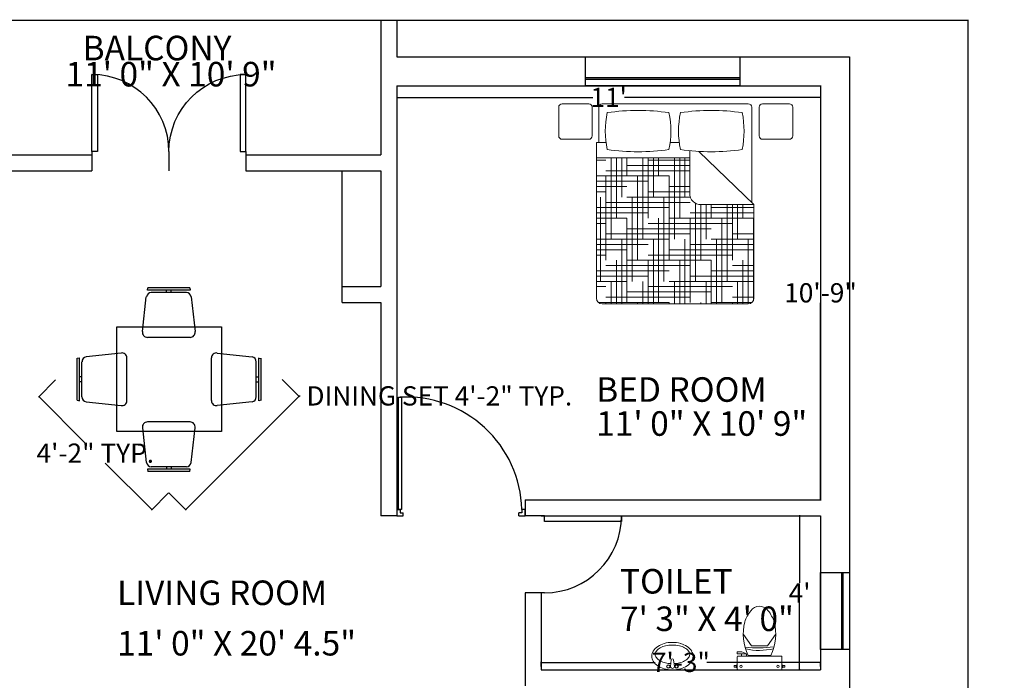
# Model space of a CAD drawing. Units: inches. Extents: x -113 to 5399, y -1393 to 3302.
# Tile 18 of 40: x 1779 to 2086, y 592 to 798. Entities that reach past the tile are written whole.
import ezdxf

# ---------------------------------------------------------------- set-up
doc = ezdxf.new("R2010")
doc.units = ezdxf.units.IN
doc.header["$MEASUREMENT"] = 0
for name, color, linetype, lineweight in [('A-ANNO-DIMS', 254, 'Continuous', 18), ('A-AREA-IDEN', 4, 'Continuous', 18), ('A-FLOR-FIXT', 8, 'Continuous', 18), ('doors', 2, 'Continuous', 25), ('furniture', 131, 'Continuous', 18), ('walls', 1, 'Continuous', 25), ('windows', 3, 'Continuous', 25)]:
    doc.layers.add(name, color=color, linetype=linetype, lineweight=lineweight)
doc.layers.add('B-FURNITURE', color=22, linetype='Continuous')
doc.styles.get("Standard").update_dxf_attribs({"font": 'arial.ttf'})
doc.dimstyles.get("Standard").update_dxf_attribs({"dimtxt": 6, "dimasz": 0.18, "dimexe": 0.18, "dimexo": 0.0625, "dimgap": 0.09, "dimtad": 0, "dimtih": 1, "dimtoh": 1, "dimdec": 1, "dimzin": 0, "dimdsep": 46, "dimlunit": 4, "dimtxsty": 'Standard', "dimblk": 'ARCHTICK', "dimcen": 0.09, "dimadec": 0, "dimazin": 0, "dimtfac": 1, "dimtdec": 1, "dimtofl": 0, "dimtmove": 0, "dimatfit": 3, "dimfxl": 1, "dimtolj": 1, "dimtzin": 0, "dimarcsym": 0})

# ---------------------------------------------------------------- blocks, each defined once
blk = doc.blocks.new('*U2')
for p, q in [((0, 0), (0, -6)), ((24, 0), (24, -6))]:
    blk.add_line(p, q)
blk.add_lwpolyline([(0, 0), (0, 24), (1.75, 24), (1.75, 0)], close=True)
blk.add_arc((0, 0), 24, 0, 90)
blk = doc.blocks.new('*X4')
at = {"color": 0}
for p, q in [((4.3594, 18.5625), (4.3594, 18.6457)), ((4.5, 18), (4.5, 18.6457)), ((4.5469, 18.1875), (4.5469, 18.6457)), ((4.5938, 18.375), (4.5938, 18.6457)), ((4.6406, 18.5625), (4.6406, 18.6457)), ((4.6875, 18.6094), (5.4375, 18.6094)), ((4.7812, 18), (4.7812, 18.6457)), ((4.8281, 18.1875), (4.8281, 18.6457)), ((4.875, 18.375), (4.875, 18.6457)), ((4.9219, 18.5625), (4.9219, 18.6457)), ((5.0625, 18), (5.0625, 18.6457)), ((5.1094, 18.1875), (5.1094, 18.6457)), ((5.1562, 18.375), (5.1562, 18.6457)), ((5.2031, 18.5625), (5.2031, 18.6457)), ((5.3438, 18), (5.3438, 18.6457)), ((5.3906, 18.1875), (5.3906, 18.6457)), ((5.4375, 18.375), (5.4375, 18.6457)), ((5.4844, 18.5625), (5.4844, 18.6457)), ((5.625, 18), (5.625, 18.6287)), ((4.3395, 18.5156), (5.0625, 18.5156)), ((4.4531, 17.8169), (4.4531, 18.5625)), ((4.5, 18.5625), (5.25, 18.5625)), ((4.7344, 17.8125), (4.7344, 18.5625)), ((5.0156, 17.8125), (5.0156, 18.5625)), ((5.2969, 17.8125), (5.2969, 18.5625)), ((5.4375, 18.5156), (5.6375, 18.5156)), ((5.5781, 17.8125), (5.5781, 18.5625)), ((5.625, 18.5625), (5.6375, 18.5625)), ((4.3395, 18.4688), (4.875, 18.4688)), ((4.3395, 18.4219), (4.6875, 18.4219)), ((5.0625, 18.4219), (5.6375, 18.4219)), ((5.25, 18.4688), (5.6375, 18.4688)), ((4.3395, 18.375), (4.5, 18.375)), ((4.4062, 17.8169), (4.4062, 18.375)), ((4.6875, 17.8114), (4.6875, 18.375)), ((4.6875, 18.3281), (5.4375, 18.3281)), ((4.875, 18.375), (5.625, 18.375)), ((4.9688, 17.625), (4.9688, 18.375)), ((5.25, 17.625), (5.25, 18.375)), ((5.5312, 17.625), (5.5312, 18.375)), ((4.3395, 18.2344), (5.0625, 18.2344)), ((4.5, 18.2812), (5.25, 18.2812)), ((5.4375, 18.2344), (5.6375, 18.2344)), ((5.625, 18.2812), (5.6375, 18.2812)), ((4.3395, 18.1875), (4.875, 18.1875)), ((4.3395, 18.1406), (4.6875, 18.1406)), ((4.3594, 17.8169), (4.3594, 18.1875)), ((4.6406, 17.8169), (4.6406, 18.1875)), ((4.9219, 17.4375), (4.9219, 18.1875)), ((5.0625, 18.1406), (5.6375, 18.1406)), ((5.2031, 17.4375), (5.2031, 18.1875)), ((5.25, 18.1875), (5.6375, 18.1875)), ((5.4844, 17.4375), (5.4844, 18.1875)), ((4.3395, 18.0938), (4.5, 18.0938)), ((4.6875, 18.0469), (5.4375, 18.0469)), ((4.875, 18.0938), (5.625, 18.0938)), ((4.5, 18), (5.25, 18)), ((4.5938, 17.8169), (4.5938, 18)), ((4.875, 17.25), (4.875, 18)), ((5.1562, 17.25), (5.1562, 18)), ((5.4375, 17.25), (5.4375, 18)), ((5.625, 18), (5.6375, 18)), ((4.3395, 17.9531), (5.0625, 17.9531)), ((4.3395, 17.9062), (4.875, 17.9062)), ((5.25, 17.9062), (5.6375, 17.9062)), ((5.4375, 17.9531), (5.6375, 17.9531)), ((4.3395, 17.8594), (4.6875, 17.8594)), ((4.8281, 17.2457), (4.8281, 17.8125)), ((4.875, 17.8125), (5.625, 17.8125)), ((5.0625, 17.8594), (5.6375, 17.8594)), ((5.1094, 17.2457), (5.1094, 17.8125)), ((5.3906, 17.2457), (5.3906, 17.8125)), ((4.7421, 17.7656), (5.4375, 17.7656)), ((4.7548, 17.7188), (5.25, 17.7188)), ((5.625, 17.7188), (5.6375, 17.7188)), ((4.7548, 17.6719), (5.0625, 17.6719)), ((4.7548, 17.625), (4.875, 17.625)), ((4.7812, 17.2457), (4.7812, 17.625)), ((5.0625, 17.2457), (5.0625, 17.625)), ((5.25, 17.625), (5.6375, 17.625)), ((5.3438, 17.2457), (5.3438, 17.625)), ((5.4375, 17.6719), (5.6375, 17.6719)), ((5.625, 17.2627), (5.625, 17.625)), ((4.875, 17.5312), (5.625, 17.5312)), ((5.0625, 17.5781), (5.6375, 17.5781)), ((4.7548, 17.4844), (5.4375, 17.4844)), ((4.7548, 17.4375), (5.25, 17.4375)), ((5.0156, 17.2457), (5.0156, 17.4375)), ((5.2969, 17.2457), (5.2969, 17.4375)), ((5.5781, 17.2457), (5.5781, 17.4375)), ((5.625, 17.4375), (5.6375, 17.4375)), ((4.7548, 17.3906), (5.0625, 17.3906)), ((4.7548, 17.3438), (4.875, 17.3438)), ((5.25, 17.3438), (5.6375, 17.3438)), ((5.4375, 17.3906), (5.6375, 17.3906)), ((5.0625, 17.2969), (5.6375, 17.2969)), ((4.875, 17.25), (5.6077, 17.25)), ((4.9688, 17.2457), (4.9688, 17.25)), ((5.25, 17.2457), (5.25, 17.25)), ((5.5312, 17.2457), (5.5312, 17.25))]:
    blk.add_line(p, q, dxfattribs=at)
blk = doc.blocks.new('MAT-P01')
for p, q in [((-0.0213, 0.8164), (-0.0213, 0.5605)), ((0.0087, 0.8464), (0.2471, 0.8464)), ((0.2771, 0.8164), (0.2771, 0.5605)), ((0.3437, 0.8164), (0.3437, -0.0316)), ((0.3737, 0.8464), (1.6737, 0.8464)), ((1.7037, 0.8164), (1.7037, 0.5005)), ((1.7622, 0.8164), (1.7622, 0.5605)), ((1.7922, 0.8464), (2.0306, 0.8464)), ((2.0606, 0.8164), (2.0606, 0.5605)), ((0.0087, 0.5305), (0.2471, 0.5305)), ((1.7922, 0.5305), (2.0306, 0.5305)), ((0.9879, 0.5005), (1.0693, 0.5005)), ((1.6393, 0.5005), (1.7237, 0.5005)), ((1.7237, 0.5005), (1.7237, -0.8836)), ((0.8146, 0.423), (0.3237, -0.0509)), ((0.8949, 0.4293), (0.8949, 0.0491)), ((0.8949, 0.3643), (1.7237, 0.3643)), ((0.8949, 0.3643), (0.8949, 0.0491)), ((0.8949, 0.3643), (1.7237, 0.3643)), ((1.7237, 0.3643), (1.7237, -0.8836)), ((0.3237, -0.0509), (0.7949, -0.0509)), ((0.3237, -0.0509), (0.3237, -0.8836)), ((0.3737, -0.9336), (1.6737, -0.9336))]:
    blk.add_line(p, q)
for centre, radius, start, end in [((0.0087, 0.8164), 0.03, 90, 180), ((0.2471, 0.8164), 0.03, 0, 90), ((0.3737, 0.8164), 0.03, 90, 180), ((1.6737, 0.8164), 0.03, 0, 90), ((1.7922, 0.8164), 0.03, 90, 180), ((2.0306, 0.8164), 0.03, 0, 90), ((1.2251, 0.6034), 0.8138, 168.37298, 191.62702), ((0.7029, -1.1436), 1.9306, 81.81622, 98.18378), ((0.1806, 0.6034), 0.8138, 348.37298, 11.62702), ((1.8766, 0.6034), 0.8138, 168.37298, 191.62702), ((1.3543, -1.1436), 1.9306, 81.81622, 98.18378), ((0.8321, 0.6034), 0.8138, 348.37298, 11.62702), ((0.0087, 0.5605), 0.03, 180, 270), ((0.2471, 0.5605), 0.03, 270, 0), ((1.7922, 0.5605), 0.03, 180, 270), ((2.0306, 0.5605), 0.03, 270, 0), ((0.7029, 2.3504), 1.9306, 261.81622, 278.18378), ((1.3543, 2.3504), 1.9306, 261.81622, 278.18378), ((0.7949, 0.0491), 0.1, 270, 0), ((0.3737, -0.8836), 0.05, 180, 270), ((1.6737, -0.8836), 0.05, 270, 0)]:
    blk.add_arc(centre, radius, start, end)
at = {"rotation": 270}
blk.add_blockref('*X4', (-16.9221, 4.7038), dxfattribs=at)
blk = doc.blocks.new('A$C6ACA79D1')
at = {"layer": 'B-FURNITURE'}
for p, q in [((-0.5034, 0.0535), (-0.8012, -0.2442)), ((-0.4835, 0.0392), (-0.7869, -0.2642)), ((-0.5034, 0.0535), (-0.4835, 0.0392)), ((-0.4291, 0.0003), (-0.1547, -0.2204)), ((0.7869, -0.259), (0.4835, 0.0444)), ((0.4842, 0.0434), (0.5041, 0.0577)), ((0.7427, -0.249), (0.4935, 0.0002)), ((0.8012, -0.239), (0.5034, 0.0587)), ((-0.4935, -0.005), (-0.7427, -0.2542)), ((-0.601, -0.1125), (-0.6181, -0.0954)), ((0.601, -0.1073), (0.6181, -0.0902)), ((-0.6352, -0.1467), (-0.6523, -0.1296)), ((0.6352, -0.1415), (0.6523, -0.1244)), ((-0.7859, -0.2635), (-0.8002, -0.2436)), ((0.4513, -0.594), (0.1485, -0.2912)), ((0.8012, -0.239), (0.7869, -0.259)), ((-0.1485, -0.2964), (-0.4513, -0.5992)), ((0.748, -0.3133), (0.5273, -0.5877)), ((-0.1485, -1.1937), (-0.4513, -0.8909)), ((0.4513, -0.8961), (0.1485, -1.199)), ((0.748, -1.1768), (0.5273, -0.9024)), ((-0.5034, -1.5436), (-0.8012, -1.2459)), ((-0.7859, -1.2266), (-0.8002, -1.2466)), ((-0.4835, -1.5293), (-0.7869, -1.226)), ((-0.4935, -1.4851), (-0.7427, -1.236)), ((-0.4291, -1.4904), (-0.1547, -1.2698)), ((0.7869, -1.2312), (0.4835, -1.5346)), ((0.7427, -1.2412), (0.4935, -1.4903)), ((0.8012, -1.2511), (0.5034, -1.5488)), ((0.8012, -1.2511), (0.7869, -1.2312)), ((-0.6352, -1.3434), (-0.6523, -1.3605)), ((-0.601, -1.3776), (-0.6181, -1.3948)), ((0.6352, -1.3486), (0.6523, -1.3657)), ((0.601, -1.3829), (0.6181, -1.4)), ((-0.5034, -1.5436), (-0.4835, -1.5293)), ((0.4842, -1.5336), (0.5041, -1.5478))]:
    blk.add_line(p, q, dxfattribs=at)
at = {"layer": 'B-FURNITURE', "ltscale": 300}
for p, q in [((0.1547, -0.2152), (0.4291, 0.0055)), ((-0.5273, -0.593), (-0.748, -0.3186)), ((-0.5273, -0.8972), (-0.748, -1.1716)), ((0.1547, -1.275), (0.4291, -1.4956))]:
    blk.add_line(p, q, dxfattribs=at)
blk.add_lwpolyline([(-0.7425, -0.7425), (0, 0), (0.7425, -0.7425), (0, -1.4849)], close=True, dxfattribs=at)
at = {"layer": 'B-FURNITURE', "ltscale": 400}
for centre, start, end in [((-0.4582, -0.0403), 54.40695, 135), ((0.4589, -0.0361), 45, 125.59305), ((-0.7063, -0.2888), 135, 215.59305), ((0.7073, -0.2843), 324.40695, 45), ((-0.7063, -1.2013), 144.40695, 225), ((0.7073, -1.2059), 315, 35.59305), ((-0.4582, -1.4498), 225, 305.59305), ((0.4589, -1.454), 234.40695, 315)]:
    blk.add_arc(centre, 0.0499, start, end, dxfattribs=at)
at = {"layer": 'B-FURNITURE', "ltscale": 300}
for centre, start, end in [((-0.1838, -0.261), 315, 54.40695), ((0.1838, -0.2558), 125.59305, 225), ((0.4866, -0.5586), 225, 324.40695), ((-0.4866, -0.5639), 215.59305, 315), ((-0.4866, -0.9263), 45, 144.40695), ((0.4866, -0.9315), 35.59305, 135), ((-0.1838, -1.2291), 305.59305, 45), ((0.1838, -1.2343), 135, 234.40695)]:
    blk.add_arc(centre, 0.05, start, end, dxfattribs=at)
blk = doc.blocks.new('toilet-3')
at = {"color": 0, "linetype": 'ByBlock'}
for p, q in [((-0.281, -0.05), (-0.281, -0.069)), ((-0.281, -0.05), (-0.261, -0.05)), ((-0.281, -0.069), (-0.261, -0.069)), ((-0.261, -0.047), (-0.261, -0.072)), ((-0.261, -0.047), (-0.251, -0.047)), ((-0.261, -0.072), (-0.251, -0.072)), ((-0.251, -0.047), (-0.251, -0.072)), ((-0.25, -0.03), (-0.25, -0.165)), ((0.24, -0.02), (-0.24, -0.02)), ((0.25, -0.03), (0.25, -0.165)), ((0.261, -0.047), (0.251, -0.047)), ((0.251, -0.047), (0.251, -0.072)), ((0.261, -0.072), (0.251, -0.072)), ((0.261, -0.047), (0.261, -0.072)), ((0.281, -0.05), (0.261, -0.05)), ((0.281, -0.069), (0.261, -0.069)), ((0.281, -0.05), (0.281, -0.069)), ((-0.144, -0.2), (-0.25, -0.2)), ((-0.25, -0.2), (-0.25, -0.222)), ((0.24, -0.175), (-0.24, -0.175)), ((-0.202, -0.2), (-0.202, -0.175)), ((-0.198, -0.222), (-0.16, -0.207)), ((-0.16, -0.207), (-0.16, -0.2)), ((-0.144, -0.2), (-0.144, -0.175)), ((0.125, -0.182), (-0.125, -0.182)), ((-0.198, -0.222), (-0.25, -0.222)), ((-0.089, -0.287), (-0.18, -0.415)), ((0.089, -0.287), (-0.089, -0.287)), ((0.089, -0.287), (0.18, -0.415))]:
    blk.add_line(p, q, dxfattribs=at)
for centre in [(-0.205, -0.059), (0.205, -0.059)]:
    blk.add_circle(centre, 0.0125, dxfattribs=at)
for centre, radius, start, end in [((-0.24, -0.03), 0.01, 90, 180), ((0.24, -0.03), 0.01, 0, 90), ((-0.24, -0.165), 0.01, 180, 270), ((0.376, -0.424), 0.557, 154.2321, 193.6755), ((-0.376, -0.424), 0.557, 346.3245, 25.7679), ((0.24, -0.165), 0.01, 270, 0), ((-0.013, -1.787), 1.521, 83.4552, 95.5271), ((-0.005, -0.896), 0.659, 75.9276, 103.0204), ((0.262, -0.406), 0.452, 199.2942, 217.2549), ((-0.265, -0.4), 0.457, 322.2382, 340.1051), ((-0.001, -0.609), 0.12, 216.3794, 323.6206)]:
    blk.add_arc(centre, radius, start, end, dxfattribs=at)
blk = doc.blocks.new('wash-6')
at = {"color": 0, "linetype": 'ByBlock'}
for p, q in [((-0.036, -0.063), (-0.021, -0.18)), ((0.036, -0.063), (0.021, -0.18))]:
    blk.add_line(p, q, dxfattribs=at)
for centre, radius in [((-0.075, -0.062), 0.0325), ((-0.075, -0.062), 0.0263), ((0.075, -0.062), 0.0325), ((0.075, -0.062), 0.0263)]:
    blk.add_circle(centre, radius, dxfattribs=at)
for centre, radius, start, end in [((0, -0.56), 0.56, 90, 105.4371), ((-0.204, -0.25), 0.17, 148.1465, 180), ((-0.107, -0.311), 0.285, 123.6901, 148.1465), ((-0.114, -0.361), 0.225, 118.369, 142.5096), ((-0.042, -0.407), 0.401, 105.4371, 123.6901), ((-0.045, -0.488), 0.37, 102.6081, 118.369), ((0, -0.69), 0.576, 92.9466, 102.6081), ((0, -0.063), 0.0361, 0, 180), ((0, -0.56), 0.56, 74.5629, 90), ((0, -0.69), 0.576, 77.3919, 87.0534), ((0.045, -0.488), 0.37, 61.631, 77.3919), ((0.042, -0.407), 0.401, 56.3099, 74.5629), ((0.114, -0.361), 0.225, 37.4904, 61.631), ((0.107, -0.311), 0.285, 31.8535, 56.3099), ((0.204, -0.25), 0.17, 0, 31.8535), ((-0.204, -0.25), 0.17, 180, 211.8535), ((-0.107, -0.189), 0.285, 211.8535, 236.3099), ((-0.217, -0.282), 0.0954, 142.5096, 180), ((-0.217, -0.282), 0.0954, 180, 217.4904), ((-0.114, -0.203), 0.225, 217.4904, 241.631), ((0, -0.18), 0.0215, 180, 0), ((0.114, -0.203), 0.225, 298.369, 322.5096), ((0.107, -0.189), 0.285, 303.6901, 328.1465), ((0.217, -0.282), 0.0954, 0, 37.4904), ((0.217, -0.282), 0.0954, 322.5096, 0), ((0.204, -0.25), 0.17, 328.1465, 0), ((-0.042, -0.092), 0.401, 236.3099, 254.5629), ((-0.045, -0.076), 0.37, 241.631, 257.3919), ((0, 0.06), 0.56, 254.5629, 270), ((0, 0.125), 0.576, 257.3919, 270), ((0, 0.125), 0.576, 270, 282.6081), ((0, 0.06), 0.56, 270, 285.4371), ((0.045, -0.076), 0.37, 282.6081, 298.369), ((0.042, -0.092), 0.401, 285.4371, 303.6901)]:
    blk.add_arc(centre, radius, start, end, dxfattribs=at)
blk = doc.blocks.new('_ArchTick')
at = {"color": 0, "linetype": 'ByBlock', "const_width": 0.15}
blk.add_lwpolyline([(-0.5, -0.5), (0.5, 0.5)], dxfattribs=at)
blk = doc.blocks.new('*D49')
at = {"layer": 'A-ANNO-DIMS', "color": 0, "lineweight": -2, "transparency": 16777216}
for p, q in [((2025.46, 777.53), (2028.44, 777.53)), ((2028.26, 777.53), (2028.26, 716.19)), ((2028.26, 648.53), (2028.26, 709.88)), ((2025.46, 648.53), (2028.44, 648.53))]:
    blk.add_line(p, q, dxfattribs=at)
at = {"layer": 'Defpoints', "color": 0, "transparency": 16777216}
for p in [(2025.39, 777.53), (2025.39, 648.53), (2028.26, 648.53)]:
    blk.add_point(p, dxfattribs=at)
at = {"layer": 'A-ANNO-DIMS', "color": 0, "lineweight": -2, "transparency": 16777216, "xscale": 0.18, "yscale": 0.18, "zscale": 0.18}
for p, rotation in [((2028.26, 777.53), 90), ((2028.26, 648.53), 270)]:
    blk.add_blockref('_ArchTick', p, dxfattribs=dict(at, rotation=rotation))
at = {"layer": 'A-ANNO-DIMS', "color": 0, "transparency": 16777216, "insert": (2028.26, 713.03), "char_height": 6, "attachment_point": 5}
blk.add_mtext('\\A1;10\'-9"', dxfattribs=at)
blk = doc.blocks.new('*D50')
at = {"layer": 'A-ANNO-DIMS', "color": 0, "lineweight": -2, "transparency": 16777216}
for p, q in [((1896.26, 773.9), (1957.36, 773.9)), ((1896.26, 773.84), (1896.26, 773.72)), ((2028.26, 773.9), (1967.16, 773.9)), ((2028.26, 773.96), (2028.26, 774.08))]:
    blk.add_line(p, q, dxfattribs=at)
at = {"layer": 'Defpoints', "color": 0, "transparency": 16777216}
for p in [(1896.26, 773.9), (2028.26, 773.9), (2028.26, 773.9)]:
    blk.add_point(p, dxfattribs=at)
at = {"layer": 'A-ANNO-DIMS', "color": 0, "lineweight": -2, "transparency": 16777216, "xscale": 0.18, "yscale": 0.18, "zscale": 0.18, "rotation": 180}
blk.add_blockref('_ArchTick', (1896.26, 773.9), dxfattribs=at)
at = {"layer": 'A-ANNO-DIMS', "color": 0, "lineweight": -2, "transparency": 16777216, "xscale": 0.18, "yscale": 0.18, "zscale": 0.18}
blk.add_blockref('_ArchTick', (2028.26, 773.9), dxfattribs=at)
at = {"layer": 'A-ANNO-DIMS', "color": 0, "transparency": 16777216, "insert": (1962.26, 773.9), "char_height": 6, "attachment_point": 5}
blk.add_mtext("\\A1;11'", dxfattribs=at)
blk = doc.blocks.new('*D51')
at = {"layer": 'A-ANNO-DIMS', "color": 0, "lineweight": -2, "transparency": 16777216}
for p, q in [((2021.92, 643.53), (2021.57, 643.53)), ((2021.75, 643.53), (2021.75, 622.62)), ((2021.75, 595.53), (2021.75, 616.44)), ((2021.92, 595.53), (2021.57, 595.53))]:
    blk.add_line(p, q, dxfattribs=at)
at = {"layer": 'Defpoints', "color": 0, "transparency": 16777216}
for p in [(2021.98, 643.53), (2021.75, 595.53), (2021.98, 595.53)]:
    blk.add_point(p, dxfattribs=at)
at = {"layer": 'A-ANNO-DIMS', "color": 0, "lineweight": -2, "transparency": 16777216, "xscale": 0.18, "yscale": 0.18, "zscale": 0.18}
for p, rotation in [((2021.75, 643.53), 90), ((2021.75, 595.53), 270)]:
    blk.add_blockref('_ArchTick', p, dxfattribs=dict(at, rotation=rotation))
at = {"layer": 'A-ANNO-DIMS', "color": 0, "transparency": 16777216, "insert": (2021.75, 619.53), "char_height": 6, "attachment_point": 5}
blk.add_mtext("\\A1;4'", dxfattribs=at)
blk = doc.blocks.new('*D54')
at = {"layer": 'A-ANNO-DIMS', "color": 0, "lineweight": -2, "transparency": 16777216}
for p, q in [((1941.26, 596.55), (1941.26, 598.06)), ((1941.26, 597.88), (1976.72, 597.88)), ((2028.26, 597.88), (1992.8, 597.88)), ((2028.26, 596.55), (2028.26, 598.06))]:
    blk.add_line(p, q, dxfattribs=at)
at = {"layer": 'Defpoints', "color": 0, "transparency": 16777216}
for p in [(1941.26, 597.88), (1941.26, 596.49), (2028.26, 596.49)]:
    blk.add_point(p, dxfattribs=at)
at = {"layer": 'A-ANNO-DIMS', "color": 0, "lineweight": -2, "transparency": 16777216, "xscale": 0.18, "yscale": 0.18, "zscale": 0.18, "rotation": 180}
blk.add_blockref('_ArchTick', (1941.26, 597.88), dxfattribs=at)
at = {"layer": 'A-ANNO-DIMS', "color": 0, "lineweight": -2, "transparency": 16777216, "xscale": 0.18, "yscale": 0.18, "zscale": 0.18}
blk.add_blockref('_ArchTick', (2028.26, 597.88), dxfattribs=at)
at = {"layer": 'A-ANNO-DIMS', "color": 0, "transparency": 16777216, "insert": (1984.76, 597.88), "char_height": 6, "attachment_point": 5}
blk.add_mtext('\\A1;7\'-3"', dxfattribs=at)
blk = doc.blocks.new('WIN-PLAN-48IN')
h = blk.add_hatch(color=256)
h.dxf.hatch_style = 1
h.paths.add_polyline_path([(48, 2.5), (0, 2.5), (0, 2), (48, 2)])
for p, q in [((0, 9), (48, 9)), ((0, 0), (0, 9)), ((48, 9), (48, 0)), ((48, 2.5), (0, 2.5)), ((48, 2), (0, 2)), ((48, 0), (0, 0))]:
    blk.add_line(p, q)
blk = doc.blocks.new('WIN-PLAN-24IN')
h = blk.add_hatch(color=256)
h.dxf.hatch_style = 1
h.paths.add_polyline_path([(6.5, 24), (6.5, 0), (7, 0), (7, 24)])
for p, q in [((0, 0), (0, 24)), ((0, 24), (9, 24)), ((6.5, 24), (6.5, 0)), ((7, 24), (7, 0)), ((9, 24), (9, 0)), ((9, 0), (0, 0))]:
    blk.add_line(p, q)
blk = doc.blocks.new('DOOR-SINGLE-36IN-PLAN')
for p, q in [((0.5, 2), (0.5, 36.98)), ((0.5, 36.98), (1.5, 36.98)), ((1.5, 36.98), (1.5, 2)), ((0, 2), (0, 0)), ((0, 2), (1.04, 2)), ((1.5, 2), (0.5, 2)), ((1.04, 2), (1.04, 0.98)), ((1.04, 0.98), (2, 0.98)), ((2, 0), (2, 0.98)), ((38.96, 0.98), (38, 0.98)), ((38, 0), (38, 0.98)), ((40, 2), (38.96, 2)), ((38.96, 2), (38.96, 0.98)), ((40, 0), (40, 2)), ((0, 0), (2, 0)), ((0, 0), (2, 0)), ((38, 0), (40, 0))]:
    blk.add_line(p, q)
blk.add_arc((2.94, 0.99), 36.04, 1.6003, 93.0893)
blk = doc.blocks.new('*D183')
at = {"layer": 'A-ANNO-DIMS', "color": 0, "lineweight": -2, "transparency": 16777216}
for p, q in [((1860.57, 686.04), (1865.95, 680.66)), ((1830.51, 645.47), (1865.82, 680.79)), ((1865.82, 680.79), (1865.95, 680.91)), ((1865.95, 680.91), (1866.13, 680.91)), ((1825.26, 650.73), (1830.64, 645.35))]:
    blk.add_line(p, q, dxfattribs=at)
at = {"layer": 'Defpoints', "color": 0, "transparency": 16777216}
for p in [(1860.53, 686.08), (1865.82, 680.79), (1825.21, 650.77)]:
    blk.add_point(p, dxfattribs=at)
at = {"layer": 'A-ANNO-DIMS', "color": 0, "lineweight": -2, "transparency": 16777216, "xscale": 0.18, "yscale": 0.18, "zscale": 0.18}
for p, rotation in [((1865.82, 680.79), 44.99999999993978), ((1830.51, 645.47), 224.9999999999398)]:
    blk.add_blockref('_ArchTick', p, dxfattribs=dict(at, rotation=rotation))
at = {"layer": 'A-ANNO-DIMS', "color": 0, "transparency": 16777216, "insert": (1909.51, 680.91), "char_height": 6, "attachment_point": 5}
blk.add_mtext('\\A1;DINING SET 4\'-2" TYP.', dxfattribs=at)
blk = doc.blocks.new('*D184')
at = {"layer": 'A-ANNO-DIMS', "color": 0, "lineweight": -2, "transparency": 16777216}
for p, q in [((1789.97, 685.93), (1784.59, 680.55)), ((1784.72, 680.67), (1799.21, 666.18)), ((1819.92, 645.47), (1805.42, 659.97)), ((1825.17, 650.73), (1819.79, 645.35))]:
    blk.add_line(p, q, dxfattribs=at)
at = {"layer": 'Defpoints', "color": 0, "transparency": 16777216}
for p in [(1790.02, 685.97), (1825.21, 650.77), (1819.92, 645.47)]:
    blk.add_point(p, dxfattribs=at)
at = {"layer": 'A-ANNO-DIMS', "color": 0, "lineweight": -2, "transparency": 16777216, "xscale": 0.18, "yscale": 0.18, "zscale": 0.18}
for p, rotation in [((1784.72, 680.67), 134.9999999999397), ((1819.92, 645.47), 314.9999999999397)]:
    blk.add_blockref('_ArchTick', p, dxfattribs=dict(at, rotation=rotation))
at = {"layer": 'A-ANNO-DIMS', "color": 0, "transparency": 16777216, "insert": (1802.32, 663.07), "char_height": 6, "attachment_point": 5}
blk.add_mtext('\\A1;4\'-2" TYP.', dxfattribs=at)
blk = doc.blocks.new('*D209')
at = {"layer": 'A-ANNO-DIMS', "color": 0, "lineweight": -2, "transparency": 16777216}
for p, q in [((1754.32, 798.03), (2074.39, 798.03)), ((2074.21, 798.03), (2074.21, 467.19)), ((2074.21, 130.03), (2074.21, 460.88)), ((1754.32, 130.03), (2074.39, 130.03))]:
    blk.add_line(p, q, dxfattribs=at)
at = {"layer": 'Defpoints', "color": 0, "transparency": 16777216}
for p in [(1754.26, 798.03), (2074.21, 798.03), (1754.26, 130.03)]:
    blk.add_point(p, dxfattribs=at)
at = {"layer": 'A-ANNO-DIMS', "color": 0, "lineweight": -2, "transparency": 16777216, "xscale": 0.18, "yscale": 0.18, "zscale": 0.18}
for p, rotation in [((2074.21, 798.03), 90), ((2074.21, 130.03), 270)]:
    blk.add_blockref('_ArchTick', p, dxfattribs=dict(at, rotation=rotation))
at = {"layer": 'A-ANNO-DIMS', "color": 0, "transparency": 16777216, "insert": (2074.21, 464.03), "char_height": 6, "attachment_point": 5}
blk.add_mtext('\\A1;55\'-8"', dxfattribs=at)

msp = doc.modelspace()

# ---------------------------------------------------------------- linework, layer by layer
at = {"layer": 'walls'}
for p, q in [((1759.26, 798.03), (1891.26, 798.03)), ((1891.26, 798.03), (1891.26, 756.03)), ((1891.26, 798.03), (1896.26, 798.03)), ((1896.26, 798.03), (1896.26, 786.53)), ((1896.26, 786.53), (2037.26, 786.53)), ((2037.26, 786.53), (2037.26, 136.53)), ((1896.26, 777.53), (1896.26, 643.53)), ((1896.26, 777.53), (2028.26, 777.53)), ((2028.26, 777.53), (2028.26, 648.53)), ((1759.26, 756.03), (1801.26, 756.03)), ((1801.26, 756.03), (1801.26, 751.03)), ((1849.26, 756.03), (1891.26, 756.03)), ((1849.26, 756.03), (1849.26, 751.03)), ((1759.26, 751.03), (1801.26, 751.03)), ((1849.26, 751.03), (1891.26, 751.03)), ((1879.26, 715.03), (1879.26, 751.03)), ((1891.26, 751.03), (1891.26, 715.03)), ((1879.26, 715.03), (1891.26, 715.03)), ((1879.26, 710.03), (1879.26, 715.03)), ((1879.26, 710.03), (1891.26, 710.03)), ((1891.26, 710.03), (1891.26, 643.53)), ((1936.26, 648.53), (1936.26, 643.53)), ((1936.26, 648.53), (2028.26, 648.53)), ((1896.26, 643.53), (1891.26, 643.53)), ((1941.26, 643.53), (1936.26, 643.53)), ((1941.26, 643.53), (2028.26, 643.53)), ((2028.26, 643.53), (2028.26, 595.53)), ((1936.26, 619.53), (1936.26, 590.53)), ((1941.26, 619.53), (1936.26, 619.53)), ((1941.26, 619.53), (1941.26, 595.53)), ((1941.26, 595.53), (2028.26, 595.53))]:
    msp.add_line(p, q, dxfattribs=at)

# ---------------------------------------------------------------- block references
at = {"layer": 'A-FLOR-FIXT', "rotation": 180}
for name, p, xscale, yscale, zscale in [('toilet-3', (2009.26, 594.97), -27.95492935005888, 27.95492935005888, 27.95492935005888), ('wash-6', (1982.14, 595.53), -17.16666334294967, 17.16666334294967, 17.16666334294967)]:
    msp.add_blockref(name, p, dxfattribs=dict(at, xscale=xscale, yscale=yscale, zscale=zscale))
at = {"layer": 'doors'}
for name, p in [('*U2', (1801.26, 757.03)), ('DOOR-SINGLE-36IN-PLAN', (1896.26, 643.53))]:
    msp.add_blockref(name, p, dxfattribs=at)
at = {"layer": 'doors', "xscale": -1}
msp.add_blockref('*U2', (1849.26, 757.03), dxfattribs=at)
at = {"layer": 'doors', "rotation": 270}
msp.add_blockref('*U2', (1942.26, 643.53), dxfattribs=at)
at = {"layer": 'furniture', "xscale": -35.02364872074636, "yscale": 35.02364872074636, "zscale": 35.02364872074636}
msp.add_blockref('MAT-P01', (2018.86, 742.29), dxfattribs=at)
at = {"layer": 'furniture', "xscale": 31.0665876167328, "yscale": 31.0665876167328, "zscale": 31.0665876167328, "rotation": 314.9999999999397}
msp.add_blockref('A$C6ACA79D1', (1841.64, 702.39), dxfattribs=at)
at = {"layer": 'windows'}
for name, p in [('WIN-PLAN-48IN', (1955.08, 777.53)), ('WIN-PLAN-24IN', (2028.26, 601.91))]:
    msp.add_blockref(name, p, dxfattribs=at)

# ---------------------------------------------------------------- texts
at = {"layer": 'A-AREA-IDEN'}
for s, height, p in [('BALCONY', 7.647, (1798.38, 785.48)), ('11\' 0" X 10\' 9"', 7.6473, (1793.05, 777.33)), ('BED ROOM', 7.647, (1958.38, 679.07)), ('11\' 0" X 10\' 9"', 7.6473, (1958.38, 668.48)), ('TOILET', 7.647, (1965.8, 619.32)), ('LIVING ROOM', 7.6473, (1809.12, 615.74)), ('7\' 3" X 4\' 0"', 7.6473, (1965.8, 607.64)), ('11\' 0" X 20\' 4.5"', 7.6473, (1809.12, 600.02))]:
    msp.add_text(s, height=height, dxfattribs=at).set_placement(p)

# ---------------------------------------------------------------- dimensions: what is measured, and where the dimension line sits
at = {"layer": 'A-ANNO-DIMS'}
for base, p1, p2, override, picture, middle in [((2074.21, 798.03), (1754.26, 130.03), (1754.26, 798.03), {"dimdec": 1, "dimlfac": 1, "dimrnd": 0, "dimzin": 1, "dimdsep": 46, "dimlunit": 4, "dimfrac": 2}, '*D209', (2074.21, 464.03)), ((2028.26, 648.53), (2025.39, 777.53), (2025.39, 648.53), {"dimclrd": 0, "dimclre": 0, "dimclrt": 0}, '*D49', (2028.26, 713.03)), ((2021.75, 595.53), (2021.98, 643.53), (2021.98, 595.53), {"dimclrd": 0, "dimclre": 0, "dimclrt": 0}, '*D51', (2021.75, 619.53))]:
    dim = msp.add_linear_dim(base=base, p1=p1, p2=p2, angle=90, dimstyle='Standard', override=override, dxfattribs=at)
    dim.commit()
    dim.dimension.update_dxf_attribs({"geometry": picture, "text_midpoint": middle})
for base, p1, p2, picture, middle in [((2028.26, 773.9), (1896.26, 773.9), (2028.26, 773.9), '*D50', (1962.26, 773.9)), ((1941.26, 597.88), (2028.26, 596.49), (1941.26, 596.49), '*D54', (1984.76, 597.88))]:
    dim = msp.add_linear_dim(base=base, p1=p1, p2=p2, dimstyle='Standard', override={"dimclrd": 0, "dimclre": 0, "dimclrt": 0}, dxfattribs=at)
    dim.commit()
    dim.dimension.update_dxf_attribs({"geometry": picture, "text_midpoint": middle})
for base, p1, p2, angle, text, picture, middle in [((1865.82, 680.79), (1825.21, 650.77), (1860.53, 686.08), 45, 'DINING SET <> TYP.', '*D183', (1909.51, 680.91)), ((1819.92, 645.47), (1790.02, 685.97), (1825.21, 650.77), 315, '<> TYP.', '*D184', (1802.32, 663.07))]:
    dim = msp.add_linear_dim(base=base, p1=p1, p2=p2, angle=angle, text=text, dimstyle='Standard', override={"dimdec": 1, "dimlfac": 1, "dimrnd": 0, "dimzin": 1, "dimdsep": 46, "dimlunit": 4, "dimfrac": 2}, dxfattribs=at)
    dim.commit()
    dim.dimension.update_dxf_attribs({"geometry": picture, "text_midpoint": middle})

doc.saveas('drawing.dxf')
